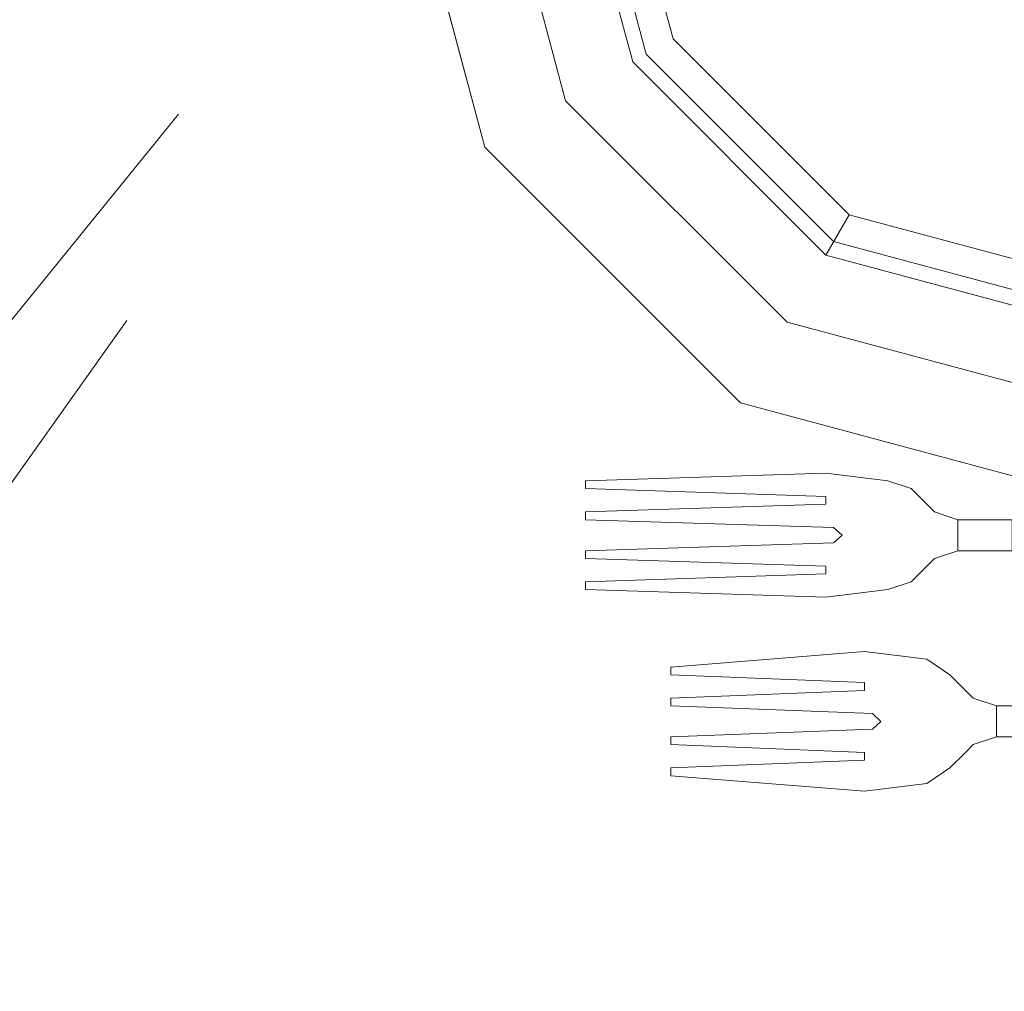
# Model space of a CAD drawing. Units: inches. Extents: x 375 to 1122, y 27 to 1069.
# Tile 106 of 155: x 731.282 to 739.094, y 859.802 to 867.512. Entities that reach past the tile are written whole.
import ezdxf

# ---------------------------------------------------------------- set-up
doc = ezdxf.new("R2010")
doc.units = ezdxf.units.IN
doc.layers.add('A-ANNO-DIMS', color=2, linetype='Continuous', lineweight=18)
doc.layers.add('Furniture', color=30, linetype='Continuous', lineweight=18)
doc.styles.get("Standard").update_dxf_attribs({"font": 'arial.ttf'})
doc.dimstyles.new('ISO-25', dxfattribs={"dimtxt": 12, "dimasz": 2.5, "dimexe": 1.5, "dimexo": 1.5, "dimtad": 1, "dimdec": 1, "dimlunit": 3, "dimtxsty": 'Standard', "dimblk": 'ARCHTICK', "dimcen": 2.5, "dimadec": 0, "dimazin": 0, "dimtfac": 1, "dimtdec": 1, "dimtmove": 0, "dimatfit": 3, "dimfxl": 1.5, "dimfxlon": 1, "dimarcsym": 0})

# ---------------------------------------------------------------- blocks, each defined once
blk = doc.blocks.new('A$C403C54AD')
for p, q in [((1.92199, 1.33837, -0.03581), (1.91891, 1.34298, -0.03534)), ((1.92199, 1.33837, -0.03888), (1.91891, 1.34298, -0.03842)), ((1.88351, 1.33067, -0.03581), (1.88197, 1.33529, -0.03534)), ((1.88351, 1.33067, -0.03888), (1.88197, 1.33529, -0.03842)), ((1.78922, 1.18993, 0.03663), (1.95298, 1.05694, 0.03663)), ((1.83016, 1.1797, 0.03663), (1.90181, 1.12855, 0.03663))]:
    blk.add_line(p, q)
at = {"linetype": 'ByBlock'}
for points, invisible_edges in [([(1.72651, 1.2691, -0.02965), (1.72651, 1.37069, -0.02965), (1.72651, 1.37069, -0.02965), (1.7773, 1.28271, -0.02965)], 5), ([(1.81449, 1.3199, -0.02965), (1.72651, 1.37069, -0.02965), (1.72651, 1.37069, -0.02965), (1.8281, 1.37069, -0.02965)], 5), ([(1.7773, 1.28271, -0.02965), (1.72651, 1.37069, -0.02965), (1.72651, 1.37069, -0.02965), (1.81449, 1.3199, -0.02965)], 5), ([(1.83048, 1.31066, -0.02349), (1.81449, 1.3199, -0.02965), (1.8281, 1.37069, -0.02965), (1.84657, 1.37069, -0.02349)], 5), ([(1.81715, 1.31836, -0.03734), (1.84648, 1.30143, -0.02811), (1.86504, 1.37069, -0.02811), (1.83118, 1.37069, -0.03734)], 5), ([(1.84648, 1.30143, -0.02349), (1.83048, 1.31066, -0.02349), (1.84657, 1.37069, -0.02349), (1.86504, 1.37069, -0.02349)], 5), ([(1.77423, 1.28804, -0.04658), (1.77884, 1.28005, -0.03734), (1.81715, 1.31836, -0.03734), (1.80916, 1.32297, -0.04658)], 1), ([(1.78654, 1.26672, -0.02349), (1.7773, 1.28271, -0.02965), (1.81449, 1.3199, -0.02965), (1.83048, 1.31066, -0.02349)], 5), ([(1.77884, 1.28005, -0.03734), (1.79578, 1.25072, -0.02811), (1.84648, 1.30143, -0.02811), (1.81715, 1.31836, -0.03734)], 5), ([(1.79578, 1.25072, -0.02349), (1.78654, 1.26672, -0.02349), (1.83048, 1.31066, -0.02349), (1.84648, 1.30143, -0.02349)], 5), ([(1.72651, 1.27526, -0.04658), (1.72651, 1.26602, -0.03734), (1.77884, 1.28005, -0.03734), (1.77423, 1.28804, -0.04658)], 5), ([(1.72651, 1.25063, -0.02349), (1.72651, 1.2691, -0.02965), (1.7773, 1.28271, -0.02965), (1.78654, 1.26672, -0.02349)], 5), ([(1.72651, 1.26602, -0.03734), (1.72651, 1.23216, -0.02811), (1.79578, 1.25072, -0.02811), (1.77884, 1.28005, -0.03734)], 5), ([(1.72651, 1.23216, -0.02349), (1.72651, 1.25063, -0.02349), (1.78654, 1.26672, -0.02349), (1.79578, 1.25072, -0.02349)], 5)]:
    blk.add_3dface(points, dxfattribs=dict(at, invisible_edges=invisible_edges))
for points in [[(1.80916, 1.32297, -0.04658), (1.81715, 1.31836, -0.03734), (1.83118, 1.37069, -0.03734), (1.82194, 1.37069, -0.04658)], [(1.84648, 1.30143, -0.02811), (1.84648, 1.30143, -0.02349), (1.86504, 1.37069, -0.02349), (1.86504, 1.37069, -0.02811)], [(1.79578, 1.25072, -0.02811), (1.79578, 1.25072, -0.02349), (1.84648, 1.30143, -0.02349), (1.84648, 1.30143, -0.02811)], [(1.72651, 1.23216, -0.02811), (1.72651, 1.23216, -0.02349), (1.79578, 1.25072, -0.02349), (1.79578, 1.25072, -0.02811)]]:
    blk.add_3dface(points, dxfattribs=at)
for points in [[(1.91275, 1.36299, -0.02863), (1.9066, 1.36299, -0.02863), (1.9066, 1.35222, -0.03071), (1.91275, 1.35222, -0.03071)], [(1.91275, 1.36299, -0.03122), (1.9066, 1.36299, -0.03122), (1.9066, 1.35222, -0.0333), (1.91275, 1.35222, -0.0333)], [(1.87581, 1.3553, -0.02863), (1.86966, 1.3553, -0.02863), (1.86966, 1.34452, -0.03071), (1.87581, 1.34452, -0.03071)], [(1.87581, 1.3553, -0.03122), (1.86966, 1.3553, -0.03122), (1.86966, 1.34452, -0.0333), (1.87581, 1.34452, -0.0333)], [(1.90352, 1.34606, -0.0341), (1.90352, 1.34606, -0.03718), (1.90044, 1.34298, -0.03842), (1.90044, 1.34298, -0.03534)], [(1.91583, 1.34606, -0.03718), (1.91583, 1.34606, -0.0341), (1.91891, 1.34298, -0.03534), (1.91891, 1.34298, -0.03842)], [(1.86658, 1.33837, -0.0341), (1.86658, 1.33837, -0.03718), (1.8635, 1.33529, -0.03842), (1.8635, 1.33529, -0.03534)], [(1.87889, 1.33837, -0.03718), (1.87889, 1.33837, -0.0341), (1.88197, 1.33529, -0.03534), (1.88197, 1.33529, -0.03842)], [(1.90968, 1.32925, -0.03868), (1.90968, 1.32925, -0.0356), (1.90814, 1.32759, -0.03545), (1.90814, 1.32759, -0.03853)], [(1.91121, 1.32759, -0.03545), (1.91121, 1.32759, -0.03853), (1.90968, 1.32925, -0.03868), (1.90968, 1.32925, -0.0356)], [(1.9066, 1.28757, -0.03119), (1.9066, 1.28757, -0.02811), (1.90814, 1.32759, -0.03545), (1.90814, 1.32759, -0.03853)], [(1.91121, 1.32759, -0.03853), (1.91121, 1.32759, -0.03545), (1.91275, 1.28757, -0.02811), (1.91275, 1.28757, -0.03119)], [(1.89582, 1.32605, -0.03829), (1.89582, 1.32605, -0.03521), (1.8989, 1.28757, -0.02811), (1.8989, 1.28757, -0.03119)], [(1.90044, 1.28757, -0.02811), (1.90044, 1.28757, -0.03119), (1.90198, 1.32605, -0.03829), (1.90198, 1.32605, -0.03521)], [(1.90352, 1.32605, -0.03829), (1.90352, 1.32605, -0.03521), (1.90198, 1.32605, -0.03521), (1.90198, 1.32605, -0.03829)], [(1.90352, 1.32605, -0.03829), (1.90352, 1.32605, -0.03521), (1.90506, 1.28757, -0.02811), (1.90506, 1.28757, -0.03119)], [(1.91429, 1.28757, -0.02811), (1.91429, 1.28757, -0.03119), (1.91583, 1.32605, -0.03829), (1.91583, 1.32605, -0.03521)], [(1.91737, 1.32605, -0.03521), (1.91737, 1.32605, -0.03829), (1.91583, 1.32605, -0.03829), (1.91583, 1.32605, -0.03521)], [(1.91737, 1.32605, -0.03521), (1.91737, 1.32605, -0.03829), (1.91891, 1.28757, -0.03119), (1.91891, 1.28757, -0.02811)], [(1.92045, 1.28757, -0.02811), (1.92045, 1.28757, -0.03119), (1.92353, 1.32605, -0.03829), (1.92353, 1.32605, -0.03521)], [(1.87273, 1.32156, -0.03868), (1.87273, 1.32156, -0.0356), (1.8712, 1.3199, -0.03545), (1.8712, 1.3199, -0.03853)], [(1.87427, 1.3199, -0.03545), (1.87427, 1.3199, -0.03853), (1.87273, 1.32156, -0.03868), (1.87273, 1.32156, -0.0356)], [(1.86966, 1.27064, -0.03119), (1.86966, 1.27064, -0.02811), (1.8712, 1.3199, -0.03545), (1.8712, 1.3199, -0.03853)], [(1.87427, 1.3199, -0.03853), (1.87427, 1.3199, -0.03545), (1.87581, 1.27064, -0.02811), (1.87581, 1.27064, -0.03119)], [(1.86042, 1.31836, -0.03829), (1.86042, 1.31836, -0.03521), (1.86196, 1.27064, -0.02811), (1.86196, 1.27064, -0.03119)], [(1.8635, 1.27064, -0.02811), (1.8635, 1.27064, -0.03119), (1.86504, 1.31836, -0.03829), (1.86504, 1.31836, -0.03521)], [(1.86658, 1.31836, -0.03829), (1.86658, 1.31836, -0.03521), (1.86504, 1.31836, -0.03521), (1.86504, 1.31836, -0.03829)], [(1.86658, 1.31836, -0.03829), (1.86658, 1.31836, -0.03521), (1.86812, 1.27064, -0.02811), (1.86812, 1.27064, -0.03119)], [(1.87735, 1.27064, -0.02811), (1.87735, 1.27064, -0.03119), (1.87889, 1.31836, -0.03829), (1.87889, 1.31836, -0.03521)], [(1.88043, 1.31836, -0.03521), (1.88043, 1.31836, -0.03829), (1.87889, 1.31836, -0.03829), (1.87889, 1.31836, -0.03521)], [(1.88043, 1.31836, -0.03521), (1.88043, 1.31836, -0.03829), (1.88197, 1.27064, -0.03119), (1.88197, 1.27064, -0.02811)], [(1.88351, 1.27064, -0.02811), (1.88351, 1.27064, -0.03119), (1.88505, 1.31836, -0.03829), (1.88505, 1.31836, -0.03521)], [(1.8989, 1.28757, -0.03119), (1.8989, 1.28757, -0.02811), (1.90044, 1.28757, -0.02811), (1.90044, 1.28757, -0.03119)], [(1.90506, 1.28757, -0.03119), (1.90506, 1.28757, -0.02811), (1.9066, 1.28757, -0.02811), (1.9066, 1.28757, -0.03119)], [(1.91275, 1.28757, -0.03119), (1.91275, 1.28757, -0.02811), (1.91429, 1.28757, -0.02811), (1.91429, 1.28757, -0.03119)], [(1.91891, 1.28757, -0.03119), (1.91891, 1.28757, -0.02811), (1.92045, 1.28757, -0.02811), (1.92045, 1.28757, -0.03119)], [(1.86196, 1.27064, -0.03119), (1.86196, 1.27064, -0.02811), (1.8635, 1.27064, -0.02811), (1.8635, 1.27064, -0.03119)], [(1.86812, 1.27064, -0.03119), (1.86812, 1.27064, -0.02811), (1.86966, 1.27064, -0.02811), (1.86966, 1.27064, -0.03119)], [(1.87581, 1.27064, -0.03119), (1.87581, 1.27064, -0.02811), (1.87735, 1.27064, -0.02811), (1.87735, 1.27064, -0.03119)], [(1.88197, 1.27064, -0.03119), (1.88197, 1.27064, -0.02811), (1.88351, 1.27064, -0.02811), (1.88351, 1.27064, -0.03119)]]:
    blk.add_3dface(points)
for points, invisible_edges in [([(1.9066, 1.36299, -0.03122), (1.9066, 1.36299, -0.02863), (1.9066, 1.35222, -0.03071), (1.9066, 1.35222, -0.0333)], 5), ([(1.91275, 1.35222, -0.0333), (1.91275, 1.35222, -0.03071), (1.91275, 1.36299, -0.02863), (1.91275, 1.36299, -0.03122)], 5), ([(1.86966, 1.3553, -0.03122), (1.86966, 1.3553, -0.02863), (1.86966, 1.34452, -0.03071), (1.86966, 1.34452, -0.0333)], 5), ([(1.87581, 1.34452, -0.0333), (1.87581, 1.34452, -0.03071), (1.87581, 1.3553, -0.02863), (1.87581, 1.3553, -0.03122)], 5), ([(1.9066, 1.35222, -0.03071), (1.91275, 1.35222, -0.03071), (1.91429, 1.3476, -0.03306), (1.90506, 1.3476, -0.03306)], 4), ([(1.9066, 1.35222, -0.0333), (1.91275, 1.35222, -0.0333), (1.91429, 1.3476, -0.03584), (1.90506, 1.3476, -0.03584)], 4), ([(1.9066, 1.35222, -0.03071), (1.9066, 1.35222, -0.0333), (1.90506, 1.3476, -0.03584), (1.90506, 1.3476, -0.03306)], 5), ([(1.91275, 1.35222, -0.0333), (1.91275, 1.35222, -0.03071), (1.91429, 1.3476, -0.03306), (1.91429, 1.3476, -0.03584)], 5), ([(1.91583, 1.34606, -0.03718), (1.90352, 1.34606, -0.03718), (1.90044, 1.34298, -0.03842), (1.91891, 1.34298, -0.03842)], 5), ([(1.91583, 1.34606, -0.0341), (1.90352, 1.34606, -0.0341), (1.90044, 1.34298, -0.03534), (1.91891, 1.34298, -0.03534)], 5), ([(1.91429, 1.3476, -0.03306), (1.90506, 1.3476, -0.03306), (1.90352, 1.34606, -0.0341), (1.91583, 1.34606, -0.0341)], 5), ([(1.91429, 1.3476, -0.03584), (1.90506, 1.3476, -0.03584), (1.90352, 1.34606, -0.03718), (1.91583, 1.34606, -0.03718)], 5), ([(1.90506, 1.3476, -0.03584), (1.90506, 1.3476, -0.03306), (1.90352, 1.34606, -0.0341), (1.90352, 1.34606, -0.03718)], 1), ([(1.91429, 1.3476, -0.03306), (1.91429, 1.3476, -0.03584), (1.91583, 1.34606, -0.03718), (1.91583, 1.34606, -0.0341)], 1), ([(1.86966, 1.34452, -0.03071), (1.87581, 1.34452, -0.03071), (1.87735, 1.33991, -0.03306), (1.86812, 1.33991, -0.03306)], 4), ([(1.86966, 1.34452, -0.03071), (1.86966, 1.34452, -0.0333), (1.86812, 1.33991, -0.03584), (1.86812, 1.33991, -0.03306)], 5), ([(1.86966, 1.34452, -0.0333), (1.87581, 1.34452, -0.0333), (1.87735, 1.33991, -0.03584), (1.86812, 1.33991, -0.03584)], 4), ([(1.87581, 1.34452, -0.0333), (1.87581, 1.34452, -0.03071), (1.87735, 1.33991, -0.03306), (1.87735, 1.33991, -0.03584)], 5), ([(1.90044, 1.34298, -0.03534), (1.91891, 1.34298, -0.03534), (1.92199, 1.33837, -0.03581), (1.89736, 1.33837, -0.03581)], 5), ([(1.90044, 1.34298, -0.03842), (1.91891, 1.34298, -0.03842), (1.92199, 1.33837, -0.03888), (1.89736, 1.33837, -0.03888)], 5), ([(1.90044, 1.34298, -0.03842), (1.90044, 1.34298, -0.03534), (1.89736, 1.33837, -0.03581), (1.89736, 1.33837, -0.03888)], 4), ([(1.91891, 1.34298, -0.03534), (1.91891, 1.34298, -0.03842), (1.92199, 1.33837, -0.03888), (1.92199, 1.33837, -0.03581)], 4), ([(1.87889, 1.33837, -0.03718), (1.86658, 1.33837, -0.03718), (1.8635, 1.33529, -0.03842), (1.88197, 1.33529, -0.03842)], 5), ([(1.87889, 1.33837, -0.0341), (1.86658, 1.33837, -0.0341), (1.8635, 1.33529, -0.03534), (1.88197, 1.33529, -0.03534)], 5), ([(1.87735, 1.33991, -0.03306), (1.86812, 1.33991, -0.03306), (1.86658, 1.33837, -0.0341), (1.87889, 1.33837, -0.0341)], 5), ([(1.87735, 1.33991, -0.03584), (1.86812, 1.33991, -0.03584), (1.86658, 1.33837, -0.03718), (1.87889, 1.33837, -0.03718)], 5), ([(1.86812, 1.33991, -0.03584), (1.86812, 1.33991, -0.03306), (1.86658, 1.33837, -0.0341), (1.86658, 1.33837, -0.03718)], 1), ([(1.87735, 1.33991, -0.03306), (1.87735, 1.33991, -0.03584), (1.87889, 1.33837, -0.03718), (1.87889, 1.33837, -0.0341)], 1), ([(1.89736, 1.33837, -0.03581), (1.90352, 1.32605, -0.03521), (1.90198, 1.32605, -0.03521), (1.89582, 1.32605, -0.03521)], 5), ([(1.89736, 1.33837, -0.03888), (1.90352, 1.32605, -0.03829), (1.90198, 1.32605, -0.03829), (1.89582, 1.32605, -0.03829)], 5), ([(1.89736, 1.33837, -0.03581), (1.89736, 1.33837, -0.03888), (1.89582, 1.32605, -0.03829), (1.89582, 1.32605, -0.03521)], 1), ([(1.89736, 1.33837, -0.03581), (1.90968, 1.32925, -0.0356), (1.90814, 1.32759, -0.03545), (1.90352, 1.32605, -0.03521)], 13), ([(1.89736, 1.33837, -0.03581), (1.90968, 1.32925, -0.0356), (1.92199, 1.33837, -0.03581), (1.89736, 1.33837, -0.03581)], 7), ([(1.89736, 1.33837, -0.03888), (1.90968, 1.32925, -0.03868), (1.90814, 1.32759, -0.03853), (1.90352, 1.32605, -0.03829)], 13), ([(1.89736, 1.33837, -0.03888), (1.90968, 1.32925, -0.03868), (1.92199, 1.33837, -0.03888), (1.89736, 1.33837, -0.03888)], 7), ([(1.92199, 1.33837, -0.03581), (1.90968, 1.32925, -0.0356), (1.91121, 1.32759, -0.03545), (1.91583, 1.32605, -0.03521)], 13), ([(1.92199, 1.33837, -0.03888), (1.90968, 1.32925, -0.03868), (1.91121, 1.32759, -0.03853), (1.91583, 1.32605, -0.03829)], 13), ([(1.92199, 1.33837, -0.03581), (1.91583, 1.32605, -0.03521), (1.91737, 1.32605, -0.03521), (1.92353, 1.32605, -0.03521)], 5), ([(1.92199, 1.33837, -0.03888), (1.91583, 1.32605, -0.03829), (1.91737, 1.32605, -0.03829), (1.92353, 1.32605, -0.03829)], 5), ([(1.92199, 1.33837, -0.03888), (1.92199, 1.33837, -0.03581), (1.92353, 1.32605, -0.03521), (1.92353, 1.32605, -0.03829)], 1), ([(1.8635, 1.33529, -0.03534), (1.88197, 1.33529, -0.03534), (1.88351, 1.33067, -0.03581), (1.86196, 1.33067, -0.03581)], 5), ([(1.8635, 1.33529, -0.03842), (1.88197, 1.33529, -0.03842), (1.88351, 1.33067, -0.03888), (1.86196, 1.33067, -0.03888)], 5), ([(1.8635, 1.33529, -0.03842), (1.8635, 1.33529, -0.03534), (1.86196, 1.33067, -0.03581), (1.86196, 1.33067, -0.03888)], 4), ([(1.88197, 1.33529, -0.03534), (1.88197, 1.33529, -0.03842), (1.88351, 1.33067, -0.03888), (1.88351, 1.33067, -0.03581)], 4), ([(1.86196, 1.33067, -0.03581), (1.86658, 1.31836, -0.03521), (1.86504, 1.31836, -0.03521), (1.86042, 1.31836, -0.03521)], 5), ([(1.86196, 1.33067, -0.03888), (1.86658, 1.31836, -0.03829), (1.86504, 1.31836, -0.03829), (1.86042, 1.31836, -0.03829)], 5), ([(1.86196, 1.33067, -0.03581), (1.86196, 1.33067, -0.03888), (1.86042, 1.31836, -0.03829), (1.86042, 1.31836, -0.03521)], 1), ([(1.86196, 1.33067, -0.03581), (1.87273, 1.32156, -0.0356), (1.8712, 1.3199, -0.03545), (1.86658, 1.31836, -0.03521)], 13), ([(1.86196, 1.33067, -0.03581), (1.87273, 1.32156, -0.0356), (1.88351, 1.33067, -0.03581), (1.86196, 1.33067, -0.03581)], 7), ([(1.86196, 1.33067, -0.03888), (1.87273, 1.32156, -0.03868), (1.88351, 1.33067, -0.03888), (1.86196, 1.33067, -0.03888)], 7), ([(1.86196, 1.33067, -0.03888), (1.87273, 1.32156, -0.03868), (1.8712, 1.3199, -0.03853), (1.86658, 1.31836, -0.03829)], 13), ([(1.88351, 1.33067, -0.03581), (1.87273, 1.32156, -0.0356), (1.87427, 1.3199, -0.03545), (1.87889, 1.31836, -0.03521)], 13), ([(1.88351, 1.33067, -0.03888), (1.87273, 1.32156, -0.03868), (1.87427, 1.3199, -0.03853), (1.87889, 1.31836, -0.03829)], 13), ([(1.88351, 1.33067, -0.03581), (1.87889, 1.31836, -0.03521), (1.88043, 1.31836, -0.03521), (1.88505, 1.31836, -0.03521)], 5), ([(1.88351, 1.33067, -0.03888), (1.87889, 1.31836, -0.03829), (1.88043, 1.31836, -0.03829), (1.88505, 1.31836, -0.03829)], 5), ([(1.88351, 1.33067, -0.03888), (1.88351, 1.33067, -0.03581), (1.88505, 1.31836, -0.03521), (1.88505, 1.31836, -0.03829)], 1), ([(1.90352, 1.32605, -0.03521), (1.90814, 1.32759, -0.03545), (1.9066, 1.28757, -0.02811), (1.90506, 1.28757, -0.02811)], 1), ([(1.90352, 1.32605, -0.03829), (1.90814, 1.32759, -0.03853), (1.9066, 1.28757, -0.03119), (1.90506, 1.28757, -0.03119)], 1), ([(1.91121, 1.32759, -0.03545), (1.91583, 1.32605, -0.03521), (1.91429, 1.28757, -0.02811), (1.91275, 1.28757, -0.02811)], 1), ([(1.91121, 1.32759, -0.03853), (1.91583, 1.32605, -0.03829), (1.91429, 1.28757, -0.03119), (1.91275, 1.28757, -0.03119)], 1), ([(1.90198, 1.32605, -0.03521), (1.89582, 1.32605, -0.03521), (1.8989, 1.28757, -0.02811), (1.90044, 1.28757, -0.02811)], 1), ([(1.90198, 1.32605, -0.03829), (1.89582, 1.32605, -0.03829), (1.8989, 1.28757, -0.03119), (1.90044, 1.28757, -0.03119)], 1), ([(1.91737, 1.32605, -0.03521), (1.92353, 1.32605, -0.03521), (1.92045, 1.28757, -0.02811), (1.91891, 1.28757, -0.02811)], 1), ([(1.91737, 1.32605, -0.03829), (1.92353, 1.32605, -0.03829), (1.92045, 1.28757, -0.03119), (1.91891, 1.28757, -0.03119)], 1), ([(1.86658, 1.31836, -0.03521), (1.8712, 1.3199, -0.03545), (1.86966, 1.27064, -0.02811), (1.86812, 1.27064, -0.02811)], 1), ([(1.86658, 1.31836, -0.03829), (1.8712, 1.3199, -0.03853), (1.86966, 1.27064, -0.03119), (1.86812, 1.27064, -0.03119)], 1), ([(1.87427, 1.3199, -0.03545), (1.87889, 1.31836, -0.03521), (1.87735, 1.27064, -0.02811), (1.87581, 1.27064, -0.02811)], 1), ([(1.87427, 1.3199, -0.03853), (1.87889, 1.31836, -0.03829), (1.87735, 1.27064, -0.03119), (1.87581, 1.27064, -0.03119)], 1), ([(1.86504, 1.31836, -0.03521), (1.86042, 1.31836, -0.03521), (1.86196, 1.27064, -0.02811), (1.8635, 1.27064, -0.02811)], 1), ([(1.86504, 1.31836, -0.03829), (1.86042, 1.31836, -0.03829), (1.86196, 1.27064, -0.03119), (1.8635, 1.27064, -0.03119)], 1), ([(1.88043, 1.31836, -0.03521), (1.88505, 1.31836, -0.03521), (1.88351, 1.27064, -0.02811), (1.88197, 1.27064, -0.02811)], 1), ([(1.88043, 1.31836, -0.03829), (1.88505, 1.31836, -0.03829), (1.88351, 1.27064, -0.03119), (1.88197, 1.27064, -0.03119)], 1)]:
    blk.add_3dface(points, dxfattribs=dict(invisible_edges=invisible_edges))
blk = doc.blocks.new('_ArchTick')
at = {"color": 0, "linetype": 'ByBlock', "const_width": 0.15}
blk.add_lwpolyline([(-0.5, -0.5), (0.5, 0.5)], dxfattribs=at)
blk = doc.blocks.new('*D85')
at = {"layer": 'A-ANNO-DIMS', "color": 0, "lineweight": -2, "transparency": 16777216}
for p, q in [((401.5073, 868.5277), (398.5073, 868.5277)), ((400.0073, 814.5277), (400.0073, 868.5277)), ((401.5073, 814.5277), (398.5073, 814.5277))]:
    blk.add_line(p, q, dxfattribs=at)
at = {"layer": 'Defpoints', "color": 0, "transparency": 16777216}
for p in [(400.0073, 868.5277), (845.0073, 868.5277), (845.0073, 814.5277)]:
    blk.add_point(p, dxfattribs=at)
at = {"layer": 'A-ANNO-DIMS', "color": 0, "lineweight": -2, "transparency": 16777216, "xscale": 2.5, "yscale": 2.5, "zscale": 2.5}
for p, rotation in [((400.0073, 868.5277), 90), ((400.0073, 814.5277), 270)]:
    blk.add_blockref('_ArchTick', p, dxfattribs=dict(at, rotation=rotation))
at = {"layer": 'A-ANNO-DIMS', "color": 0, "transparency": 16777216, "insert": (393.2555, 841.5277), "char_height": 12, "attachment_point": 5, "rotation": 90}
blk.add_mtext('4\'-6"', dxfattribs=at)
blk = doc.blocks.new('*D88')
at = {"layer": 'A-ANNO-DIMS', "color": 0, "lineweight": -2, "transparency": 16777216}
for p, q in [((731.0073, 1052.5277), (731.0073, 1055.5277)), ((854.0073, 1052.5277), (854.0073, 1055.5277)), ((731.0073, 1054.0277), (854.0073, 1054.0277))]:
    blk.add_line(p, q, dxfattribs=at)
at = {"layer": 'Defpoints', "color": 0, "transparency": 16777216}
for p in [(854.0073, 1054.0277), (731.0073, 502.5277), (854.0073, 502.5277)]:
    blk.add_point(p, dxfattribs=at)
at = {"layer": 'A-ANNO-DIMS', "color": 0, "lineweight": -2, "transparency": 16777216, "xscale": 2.5, "yscale": 2.5, "zscale": 2.5, "rotation": 180}
blk.add_blockref('_ArchTick', (731.0073, 1054.0277), dxfattribs=at)
at = {"layer": 'A-ANNO-DIMS', "color": 0, "lineweight": -2, "transparency": 16777216, "xscale": 2.5, "yscale": 2.5, "zscale": 2.5}
blk.add_blockref('_ArchTick', (854.0073, 1054.0277), dxfattribs=at)
at = {"layer": 'A-ANNO-DIMS', "color": 0, "transparency": 16777216, "insert": (792.5073, 1060.7837), "char_height": 12, "attachment_point": 5}
blk.add_mtext('10\'-3"', dxfattribs=at)
blk = doc.blocks.new('*D91')
at = {"layer": 'A-ANNO-DIMS', "color": 0, "lineweight": -2, "transparency": 16777216}
for p, q in [((728.0073, 1052.5277), (728.0073, 1055.5277)), ((788.0073, 1052.5277), (788.0073, 1055.5277)), ((728.0073, 1054.0277), (788.0073, 1054.0277))]:
    blk.add_line(p, q, dxfattribs=at)
at = {"layer": 'Defpoints', "color": 0, "transparency": 16777216}
for p in [(788.0073, 1054.0277), (728.0073, 774.0277), (788.0073, 774.0277)]:
    blk.add_point(p, dxfattribs=at)
at = {"layer": 'A-ANNO-DIMS', "color": 0, "lineweight": -2, "transparency": 16777216, "xscale": 2.5, "yscale": 2.5, "zscale": 2.5, "rotation": 180}
blk.add_blockref('_ArchTick', (728.0073, 1054.0277), dxfattribs=at)
at = {"layer": 'A-ANNO-DIMS', "color": 0, "lineweight": -2, "transparency": 16777216, "xscale": 2.5, "yscale": 2.5, "zscale": 2.5}
blk.add_blockref('_ArchTick', (788.0073, 1054.0277), dxfattribs=at)
at = {"layer": 'A-ANNO-DIMS', "color": 0, "transparency": 16777216, "insert": (758.0073, 1060.7796), "char_height": 12, "attachment_point": 5}
blk.add_mtext('5\'-0"', dxfattribs=at)

msp = doc.modelspace()

# ---------------------------------------------------------------- block references
at = {"layer": 'Furniture', "xscale": 39.9918517141215, "yscale": 39.9918517141215, "zscale": 39.9918517141215, "rotation": 270}
msp.add_blockref('A$C403C54AD', (684.9549, 938.3156, 0.024), dxfattribs=at)

# ---------------------------------------------------------------- dimensions: what is measured, and where the dimension line sits
at = {"layer": 'A-ANNO-DIMS'}
for base, p1, p2, picture, middle in [((788.0073, 1054.0277), (728.0073, 774.0277), (788.0073, 774.0277), '*D91', (758.0073, 1060.7796)), ((854.0073, 1054.0277), (731.0073, 502.5277), (854.0073, 502.5277), '*D88', (792.5073, 1060.7837))]:
    dim = msp.add_linear_dim(base=base, p1=p1, p2=p2, dimstyle='ISO-25', override={"dimdec": 1, "dimlfac": 1, "dimrnd": 0, "dimzin": 1, "dimdsep": 46, "dimlunit": 4, "dimfrac": 2}, dxfattribs=at)
    dim.commit()
    dim.dimension.update_dxf_attribs({"geometry": picture, "text_midpoint": middle})
dim = msp.add_linear_dim(base=(400.0073, 868.5277), p1=(845.0073, 814.5277), p2=(845.0073, 868.5277), angle=90, dimstyle='ISO-25', override={"dimdec": 1, "dimlfac": 1, "dimrnd": 0, "dimzin": 1, "dimdsep": 46, "dimlunit": 4, "dimfrac": 2}, dxfattribs=at)
dim.commit()
dim.dimension.update_dxf_attribs({"geometry": '*D85', "text_midpoint": (393.2555, 841.5277)})

doc.saveas('drawing.dxf')
